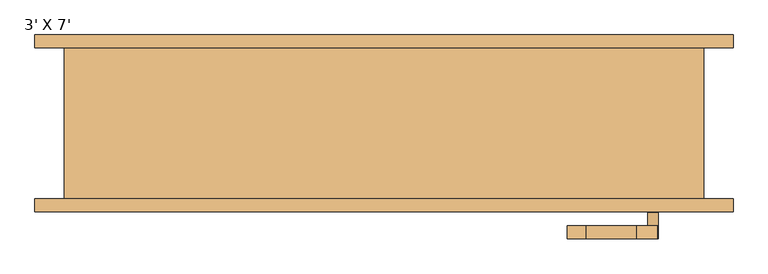
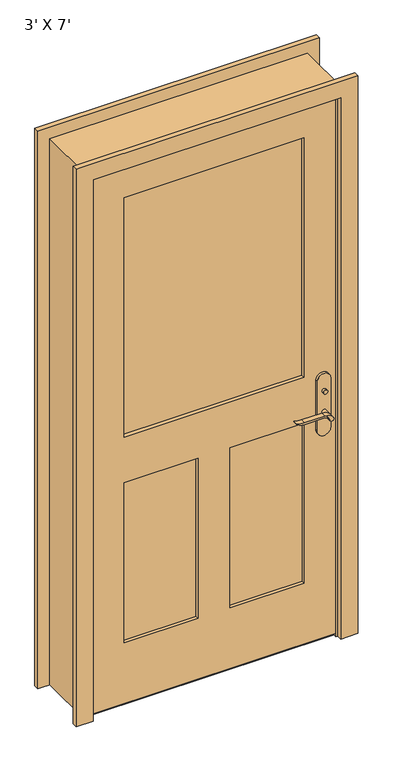
"""IFC4 building model written with IfcOpenShell, lengths in millimetres: door geometry, 3' X 7'."""

from ifc_helpers import new_model, si_unit, point, frame, frame_2d, origin, place, context, project, spatial, polyline, circle_curve, trimmed, segment, composite_curve, outline, extrude, faceted_brep, source, transform, mapped, element, save


def door_3_x_7_64fb43ed(model_context):
    return source(origin(), model_context, "Body", "SolidModel", [
        extrude(outline(polyline([(-38.1, 12.7), (-12.7, 0.0), (-98.425, 0.0), (-73.025, 12.7), (-38.1, 12.7)])), frame((-457.2, 0.0, 0.0), z_axis=(1.0, 0.0, 0.0), x_axis=(0.0, 1.0, 0.0)), (0.0, 0.0, 1.0), 914.4),
        extrude(outline(polyline([(411.4, -56.2), (411.4, -66.2), (401.4, -66.2), (401.4, -56.2), (411.4, -56.2)])), frame((0.0, 0.0, 981.9), z_axis=(0.0, 0.0, 1.0), x_axis=(1.0, 0.0, 0.0)), (0.0, 0.0, 1.0), 30.0),
        extrude(outline(composite_curve([segment(trimmed(circle_curve(frame_2d((996.9, 406.4)), 8.0), [point((996.9, 398.4))], [point((996.9, 414.4))], False, "CARTESIAN"), True, "CONTINUOUS"), segment(trimmed(circle_curve(frame_2d((996.9, 406.4)), 8.0), [point((996.9, 414.4))], [point((996.9, 398.4))], False, "CARTESIAN"), True, "CONTINUOUS")], self_intersect=False)), frame((0.0, -131.125, 0.0), z_axis=(0.0, 1.0, 0.0), x_axis=(0.0, 0.0, 1.0)), (0.0, 0.0, 1.0), 10.0),
        extrude(outline(composite_curve([segment(trimmed(circle_curve(frame_2d((897.1555521, 382.7324871)), 37.2832219), [point((919.0523287, 412.9081363))], [point((934.4, 381.0325667))], False, "CARTESIAN"), True, "CONTINUOUS"), segment(polyline([(934.4, 381.0325667), (934.4, 304.7564091)]), True, "CONTINUOUS"), segment(trimmed(circle_curve(frame_2d((1017.6850638, 304.8227909)), 83.2850902), [point((934.4, 304.7564091))], [point((939.4, 276.4))], True, "CARTESIAN"), True, "CONTINUOUS"), segment(polyline([(939.4, 276.4), (936.6135558, 276.4)]), True, "CONTINUOUS"), segment(trimmed(circle_curve(frame_2d((986.6709207, 308.3396612)), 59.3791355), [point((936.6135558, 276.4))], [point((927.4, 304.7564091))], False, "CARTESIAN"), True, "CONTINUOUS"), segment(polyline([(927.4, 304.7564091), (927.4, 381.0138099)]), True, "CONTINUOUS"), segment(trimmed(circle_curve(frame_2d((909.2738613, 381.0138099)), 18.1261387), [point((927.4, 381.0138099))], [point((914.4, 398.4))], True, "CARTESIAN"), True, "CONTINUOUS"), segment(trimmed(circle_curve(frame_2d((914.4, 406.4)), 8.0), [point((914.4, 398.4))], [point((919.0523287, 412.9081363))], False, "CARTESIAN"), True, "CONTINUOUS")], self_intersect=False)), frame((0.0, -36.2, 0.0), z_axis=(0.0, 1.0, 0.0), x_axis=(0.0, 0.0, 1.0)), (0.0, 0.0, 1.0), 20.0),
        extrude(outline(composite_curve([segment(trimmed(circle_curve(frame_2d((914.4, 406.4)), 8.0), [point((914.3999903, 398.4))], [point((919.0523287, 412.9081363))], False, "CARTESIAN"), True, "CONTINUOUS"), segment(trimmed(circle_curve(frame_2d((897.1555521, 382.7324871)), 37.2832219), [point((919.0523287, 412.9081363))], [point((934.4, 381.0325667))], False, "CARTESIAN"), True, "CONTINUOUS"), segment(polyline([(934.4, 381.0325667), (934.4, 304.7564091)]), True, "CONTINUOUS"), segment(trimmed(circle_curve(frame_2d((1017.6850638, 304.8227909)), 83.2850902), [point((934.4, 304.7564091))], [point((939.4, 276.4))], True, "CARTESIAN"), True, "CONTINUOUS"), segment(polyline([(939.4, 276.4), (936.6135558, 276.4)]), True, "CONTINUOUS"), segment(trimmed(circle_curve(frame_2d((986.6709207, 308.3396612)), 59.3791355), [point((936.6135558, 276.4))], [point((927.4, 304.7564091))], False, "CARTESIAN"), True, "CONTINUOUS"), segment(polyline([(927.4, 304.7564091), (927.4, 381.0138122)]), True, "CONTINUOUS"), segment(trimmed(circle_curve(frame_2d((909.2738682, 381.0138122)), 18.1261318), [point((927.4, 381.0138122))], [point((914.3999903, 398.4))], True, "CARTESIAN"), True, "CONTINUOUS")], self_intersect=False)), frame((0.0, -171.125, 0.0), z_axis=(0.0, 1.0, 0.0), x_axis=(0.0, 0.0, 1.0)), (0.0, 0.0, 1.0), 20.0),
        extrude(outline(composite_curve([segment(trimmed(circle_curve(frame_2d((914.4, 406.4)), 8.0), [point((914.4, 398.4))], [point((914.4, 414.4))], False, "CARTESIAN"), True, "CONTINUOUS"), segment(trimmed(circle_curve(frame_2d((914.4, 406.4)), 8.0), [point((914.4, 414.4))], [point((914.4, 398.4))], False, "CARTESIAN"), True, "CONTINUOUS")], self_intersect=False)), frame((0.0, -66.2, 0.0), z_axis=(0.0, 1.0, 0.0), x_axis=(0.0, 0.0, 1.0)), (0.0, 0.0, 1.0), 30.0),
        extrude(outline(composite_curve([segment(trimmed(circle_curve(frame_2d((914.4, 406.4)), 8.0), [point((914.4, 398.4))], [point((914.4, 414.4))], False, "CARTESIAN"), True, "CONTINUOUS"), segment(trimmed(circle_curve(frame_2d((914.4, 406.4)), 8.0), [point((914.4, 414.4))], [point((914.4, 398.4))], False, "CARTESIAN"), True, "CONTINUOUS")], self_intersect=False)), frame((0.0, -151.125, 0.0), z_axis=(0.0, 1.0, 0.0), x_axis=(0.0, 0.0, 1.0)), (0.0, 0.0, 1.0), 30.0),
        extrude(outline(composite_curve([segment(polyline([(844.4, 431.4), (1039.4, 431.4)]), True, "CONTINUOUS"), segment(trimmed(circle_curve(frame_2d((1039.4, 406.4)), 25.0), [point((1039.4, 431.4))], [point((1039.4, 381.4))], False, "CARTESIAN"), True, "CONTINUOUS"), segment(polyline([(1039.4, 381.4), (844.4, 381.4)]), True, "CONTINUOUS"), segment(trimmed(circle_curve(frame_2d((844.4, 406.4)), 25.0), [point((844.4, 381.4))], [point((844.4, 431.4))], False, "CARTESIAN"), True, "CONTINUOUS")], self_intersect=False)), frame((0.0, -76.2, 0.0), z_axis=(0.0, 1.0, 0.0), x_axis=(0.0, 0.0, 1.0)), (0.0, 0.0, 1.0), 10.0),
        extrude(outline(composite_curve([segment(polyline([(844.4, 431.4), (1039.4, 431.4)]), True, "CONTINUOUS"), segment(trimmed(circle_curve(frame_2d((1039.4, 406.4)), 25.0), [point((1039.4, 431.4))], [point((1039.4, 381.4))], False, "CARTESIAN"), True, "CONTINUOUS"), segment(polyline([(1039.4, 381.4), (844.4, 381.4)]), True, "CONTINUOUS"), segment(trimmed(circle_curve(frame_2d((844.4, 406.4)), 25.0), [point((844.4, 381.4))], [point((844.4, 431.4))], False, "CARTESIAN"), True, "CONTINUOUS")], self_intersect=False)), frame((0.0, -121.125, 0.0), z_axis=(0.0, 1.0, 0.0), x_axis=(0.0, 0.0, 1.0)), (0.0, 0.0, 1.0), 10.0),
        faceted_brep([(482.6, -111.125, 0.0), (457.2, -111.125, 0.0), (457.2, -76.2, 0.0), (444.5, -76.2, 0.0), (444.5, -41.275, 0.0), (457.2, -41.275, 0.0), (457.2, 117.475, 0.0), (482.6, 117.475, 0.0), (482.6, 117.475, 2159.0), (482.6, -111.125, 2159.0), (457.2, 117.475, 2133.6), (-457.2, 117.475, 2133.6), (-457.2, 117.475, 0.0), (-482.6, 117.475, 0.0), (-482.6, 117.475, 2159.0), (457.2, -41.275, 2133.6), (444.5, -41.275, 2120.9), (-444.5, -41.275, 2120.9), (-444.5, -41.275, 0.0), (-457.2, -41.275, 0.0), (-457.2, -41.275, 2133.6), (444.5, -76.2, 2120.9), (457.2, -76.2, 2133.6), (-457.2, -76.2, 2133.6), (-457.2, -76.2, 0.0), (-444.5, -76.2, 0.0), (-444.5, -76.2, 2120.9), (457.2, -111.125, 2133.6), (-482.6, -111.125, 2159.0), (-482.6, -111.125, 0.0), (-457.2, -111.125, 0.0), (-457.2, -111.125, 2133.6)], [[[0, 1, 2, 3, 4, 5, 6, 7]], [[7, 8, 9, 0]], [[6, 10, 11, 12, 13, 14, 8, 7]], [[5, 15, 10, 6]], [[4, 16, 17, 18, 19, 20, 15, 5]], [[3, 21, 16, 4]], [[2, 22, 23, 24, 25, 26, 21, 3]], [[1, 27, 22, 2]], [[0, 9, 28, 29, 30, 31, 27, 1]], [[8, 14, 28, 9]], [[15, 20, 11, 10]], [[21, 26, 17, 16]], [[27, 31, 23, 22]], [[29, 13, 12, 19, 18, 25, 24, 30]], [[14, 13, 29, 28]], [[20, 19, 12, 11]], [[26, 25, 18, 17]], [[31, 30, 24, 23]]]),
        extrude(outline(polyline([(2133.6, -457.2), (12.7, -457.2), (12.7, 457.2), (2133.6, 457.2), (2133.6, -457.2)]), holes=[polyline([(1066.8, -336.55), (2012.95, -336.55), (2012.95, 336.55), (1066.8, 336.55), (1066.8, -336.55)]), polyline([(885.825, -60.325), (254.0, -60.325), (254.0, -336.55), (885.825, -336.55), (885.825, -60.325)]), polyline([(885.825, 336.55), (254.0, 336.55), (254.0, 60.325), (885.825, 60.325), (885.825, 336.55)])]), frame((0.0, -111.125, 0.0), z_axis=(0.0, 1.0, 0.0), x_axis=(0.0, 0.0, 1.0)), (0.0, 0.0, 1.0), 34.925),
        extrude(outline(polyline([(336.55, -90.17), (336.55, -97.155), (-336.55, -97.155), (-336.55, -90.17), (336.55, -90.17)])), frame((0.0, 0.0, 1066.8), z_axis=(0.0, 0.0, 1.0), x_axis=(1.0, 0.0, 0.0)), (0.0, 0.0, 1.0), 946.15),
        extrude(outline(polyline([(-60.325, -87.8416667), (-60.325, -99.4833333), (-336.55, -99.4833333), (-336.55, -87.8416667), (-60.325, -87.8416667)])), frame((0.0, 0.0, 254.0), z_axis=(0.0, 0.0, 1.0), x_axis=(1.0, 0.0, 0.0)), (0.0, 0.0, 1.0), 631.825),
        extrude(outline(polyline([(336.55, -87.8416667), (336.55, -99.4833333), (60.325, -99.4833333), (60.325, -87.8416667), (336.55, -87.8416667)])), frame((0.0, 0.0, 254.0), z_axis=(0.0, 0.0, 1.0), x_axis=(1.0, 0.0, 0.0)), (0.0, 0.0, 1.0), 631.825),
        extrude(outline(polyline([(0.0, -463.55), (2139.95, -463.55), (2139.95, 463.55), (0.0, 463.55), (0.0, 527.05), (2203.45, 527.05), (2203.45, -527.05), (0.0, -527.05), (0.0, -463.55)])), frame((0.0, -130.175, 0.0), z_axis=(0.0, 1.0, 0.0), x_axis=(0.0, 0.0, 1.0)), (0.0, 0.0, 1.0), 19.05),
        extrude(outline(polyline([(0.0, -463.55), (2139.95, -463.55), (2139.95, 463.55), (0.0, 463.55), (0.0, 527.05), (2203.45, 527.05), (2203.45, -527.05), (0.0, -527.05), (0.0, -463.55)])), frame((0.0, 117.475, 0.0), z_axis=(0.0, 1.0, 0.0), x_axis=(0.0, 0.0, 1.0)), (0.0, 0.0, 1.0), 19.05),
    ])


if __name__ == "__main__":
    model = new_model("IFC4")
    model_context = context("Model", 3, world=origin())
    ifc_project = project(units=[si_unit("LENGTHUNIT", "METRE", prefix="MILLI")], contexts=[model_context])
    site = spatial("IfcSite", under=ifc_project)
    building = spatial("IfcBuilding", under=site)
    placement = place(None, origin())
    door_3_x_7_shape = door_3_x_7_64fb43ed(model_context)
    element("IfcDoor", 1, ObjectType="3' X 7'", at=placement, inside=building, context=model_context, shape_type="MappedRepresentation", body=[
        mapped(door_3_x_7_shape, transform((0.0, 0.0, 0.0), x_axis=(1.0, 0.0, 0.0), y_axis=(0.0, 1.0, 0.0), z_axis=(0.0, 0.0, 1.0))),
    ])
    save(model, "model.ifc")

# Revit data of these elements
# Type "3' X 7'"
#   Type Mark = "16"
#   Assembly Code = "B2030100"
#   Analytic Construction = "French door, wood frame with single glass"
#   Top Rail = 0' - 4 3/4"
#   Threshold Offset [instance default] = 0' - 0 1/2"
#   Thickness = 0' - 1 3/8"
#   Thermal Resistance (R) = 1.0696 (h·ft²·°F)/BTU
#   Swing Angle [instance default] = 90.00°
#   Stiles = 0' - 4 3/4"
#   Rough Width = 3' - 2"
#   Rough Height = 7' - 1"
#   Lock Rail = 0' - 7 1/8"
#   Height = 7' - 0"
#   Width = 3' - 0"
#   Heat Transfer Coefficient (U) = 0.9350 BTU/(h·ft²·°F)
#   Door Offset [instance default] = 0' - 0"
#   Bottom Rail = 0' - 9 1/2"
#   Threshold [instance default] = yes
#   Function = 1
#   Exterior Trim [instance default] = yes
#   Trim Material = Cherry
#   Threshold Material = Cherry
#   Panel Material = Cherry
#   Glazing = Glass
#   Frame Material = Cherry
#   Door Handle Material = Aluminum
#   Visual Light Transmittance = 0
#   Solar Heat Gain Coefficient = 0
#   Wall Closure = (empty or 0)
#   Construction Type = (empty or 0)
# Element 1 (IfcDoor, "3' X 7'")
#   Materials on its faces: "Cherry", "Aluminum", "Glass"
# Materials
#   "Cherry": class "Wood", colour RGB 226 177 128, transparency 0, Description = "Prunus Serotina", Cost = 0
#   "Glass": class "Glass", colour RGB 0 128 192, transparency 0.75, Description = "Soda Lime Glass", Cost = 0
#   "Aluminum": class "Metal", colour RGB 247 247 247, transparency 0, Description = "Aluminum 6061", Cost = 0
